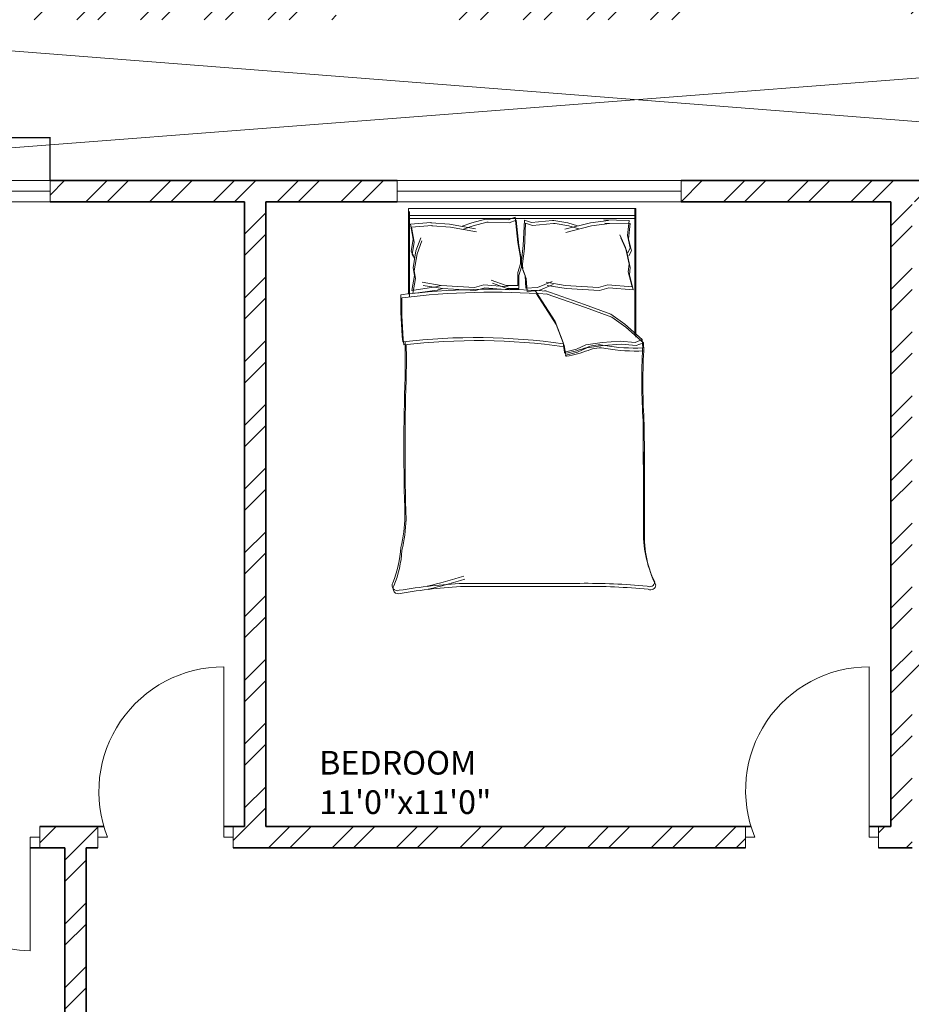
# Model space of a CAD drawing. Units: inches. Extents: x 1885 to 2748, y 783 to 2421.
# Tile 41 of 117: x 2098 to 2287, y 1350 to 1558. Entities that reach past the tile are written whole.
import ezdxf

# ---------------------------------------------------------------- set-up
doc = ezdxf.new("R2010")
doc.units = ezdxf.units.IN
for name, color, linetype, lineweight in [('A-ANNO-DIMS', 2, 'Continuous', 18), ('A-AREA-IDEN', 7, 'Continuous', 18), ('A-DOOR', 31, 'Continuous', 18), ('A-FLOR-OPEN', 8, 'Continuous', 13), ('A-FURN', 8, 'Continuous', 13), ('A-GLAZ', 181, 'Continuous', 18), ('A-WALL', 7, 'Continuous', 35)]:
    doc.layers.add(name, color=color, linetype=linetype, lineweight=lineweight)
doc.layers.add('A-WALL-PATT', color=85, linetype='Continuous', lineweight=13, true_color=0x58ba48)
doc.styles.get("Standard").update_dxf_attribs({"font": 'arial.ttf'})
doc.dimstyles.get("Standard").update_dxf_attribs({"dimtxt": 0.18, "dimasz": 0.18, "dimexe": 0.18, "dimexo": 0.0625, "dimgap": 0.09, "dimtad": 0, "dimtih": 1, "dimtoh": 1, "dimdec": 4, "dimzin": 0, "dimdsep": 46, "dimtxsty": 'Standard', "dimcen": 0.09, "dimadec": 0, "dimazin": 0, "dimtfac": 1, "dimtdec": 4, "dimtofl": 0, "dimtmove": 0, "dimatfit": 3, "dimfxl": 1, "dimtolj": 1, "dimtzin": 0, "dimarcsym": 0})

# ---------------------------------------------------------------- blocks, each defined once
blk = doc.blocks.new('BED-DOUBLE')
for p, q in [((27.75, 52.87), (24.5, 49.16)), ((27.75, 52.87), (24.5, 49.16)), ((28.39, 53.09), (25.14, 49.39)), ((28.39, 53.09), (25.14, 49.39)), ((29.49, 52.95), (27.75, 52.87, 3.87)), ((29.49, 52.95), (27.75, 52.87, 3.87)), ((28.37, 51.33), (27.75, 52.87)), ((28.37, 51.33), (27.75, 52.87)), ((30.13, 53.17), (28.39, 53.09, 3.87)), ((30.13, 53.17), (28.39, 53.09, 3.87)), ((29.01, 51.56), (28.39, 53.09)), ((29.01, 51.56), (28.39, 53.09)), ((0, 51.49), (0.64, 51.49)), ((0, 3.47), (0, 51.49)), ((0, 51.26), (26.61, 51.26)), ((0, 51.26), (26.61, 51.26)), ((0.64, 51.49), (27.25, 51.49)), ((0.64, 51.49), (27.25, 51.49)), ((1.54, 3.47), (1.54, 51.26)), ((1.54, 3.47), (1.54, 51.26)), ((2.18, 3.7), (2.18, 51.49)), ((2.18, 3.7), (2.18, 51.49)), ((2.56, 50.11), (2.46, 44.71)), ((2.56, 50.11), (2.46, 44.71)), ((2.56, 50.11), (5.77, 49.73)), ((2.56, 50.11), (5.77, 49.73)), ((3.2, 50.34), (3.1, 44.94)), ((3.2, 50.34), (3.1, 44.94)), ((3.2, 50.34), (6.41, 49.96)), ((3.2, 50.34), (6.41, 49.96)), ((5.77, 49.73), (8.34, 50.33)), ((5.77, 49.73), (8.34, 50.33)), ((6.41, 49.96), (8.98, 50.56)), ((6.41, 49.96), (8.98, 50.56)), ((11.83, 50.11), (8.26, 49.31)), ((11.83, 50.11), (8.26, 49.31)), ((8.34, 50.33), (9.39, 49.81)), ((8.34, 50.33), (9.39, 49.81)), ((12.47, 50.34), (8.9, 49.54)), ((12.47, 50.34), (8.9, 49.54)), ((8.98, 50.56), (10.03, 50.04)), ((8.98, 50.56), (10.03, 50.04)), ((13.44, 49.92), (11.83, 50.11)), ((13.44, 49.92), (11.83, 50.11)), ((14.08, 50.15), (12.47, 50.34)), ((14.08, 50.15), (12.47, 50.34)), ((16.58, 50.7), (13.44, 49.92)), ((16.58, 50.7), (13.44, 49.92)), ((17.22, 50.93), (14.08, 50.15)), ((17.22, 50.93), (14.08, 50.15)), ((16.17, 45.57), (16.58, 50.7)), ((16.17, 45.56), (16.58, 50.7)), ((16.81, 45.79), (17.22, 50.93)), ((16.81, 45.79), (17.22, 50.93)), ((28.06, 48.23), (28.37, 51.33)), ((28.06, 48.23), (28.37, 51.33)), ((28.7, 48.46), (29.01, 51.56)), ((28.7, 48.46), (29.01, 51.56)), ((8.26, 49.31), (5.58, 48.13)), ((8.26, 49.31), (5.58, 48.13)), ((8.9, 49.54), (6.22, 48.36)), ((8.9, 49.54), (6.22, 48.36)), ((24.5, 49.16), (22.33, 46.22)), ((24.5, 49.16), (22.33, 46.22)), ((25.14, 49.39), (22.97, 46.45)), ((25.14, 49.39), (22.97, 46.45)), ((28.37, 44.36), (28.06, 48.23)), ((28.37, 44.36), (28.06, 48.23)), ((29.01, 44.59), (28.7, 48.46)), ((29.01, 44.59), (28.7, 48.46)), ((3.1, 44.94), (3.19, 45.94)), ((3.1, 44.94), (3.19, 45.94)), ((3.19, 45.94), (3.71, 42.14)), ((3.19, 45.94), (3.71, 42.14)), ((17.37, 43.83), (16.81, 45.79)), ((17.37, 43.83), (16.81, 45.79)), ((22.33, 46.22), (20.32, 40.64)), ((22.33, 46.22), (20.32, 40.64)), ((22.97, 46.45), (20.96, 40.87)), ((22.97, 46.45), (20.96, 40.87)), ((2.46, 44.71), (2.55, 45.71)), ((2.46, 44.71), (2.55, 45.71)), ((2.55, 45.71), (3.07, 41.91)), ((2.55, 45.71), (3.07, 41.91)), ((16.73, 43.6), (16.17, 45.57)), ((16.73, 43.6), (16.17, 45.56)), ((16.94, 36.82), (17.37, 43.83)), ((16.94, 36.82), (17.37, 43.83)), ((28.83, 40.95), (28.37, 44.36)), ((28.83, 40.95), (28.37, 44.36)), ((29.47, 41.18), (29.01, 44.59)), ((29.47, 41.18), (29.01, 44.59)), ((3.07, 41.91), (4.43, 36.49)), ((3.07, 41.91), (4.43, 36.49)), ((3.71, 42.14), (5.07, 36.72)), ((3.71, 42.14), (5.07, 36.72)), ((16.3, 36.59), (16.73, 43.6)), ((16.3, 36.59), (16.73, 43.6)), ((20.32, 40.64), (17.39, 32.3)), ((20.32, 40.64), (17.39, 32.3)), ((20.96, 40.87), (18.03, 32.53)), ((20.96, 40.87), (18.03, 32.53)), ((29.76, 38.94), (28.83, 40.95)), ((29.76, 38.94), (28.83, 40.95)), ((30.4, 39.17), (29.47, 41.18)), ((30.4, 39.17), (29.47, 41.18)), ((79.25, 15.06), (79.25, 39.68)), ((79.25, 15.06), (79.25, 39.68)), ((79.89, 15.29), (79.89, 39.9)), ((79.89, 15.29), (79.89, 39.9)), ((3.68, 39.2), (3.08, 37.13)), ((3.68, 39.2), (3.08, 37.13)), ((4.32, 39.43), (3.72, 37.36)), ((4.32, 39.43), (3.72, 37.36)), ((30.38, 36.46), (29.76, 38.94)), ((30.38, 36.46), (29.76, 38.94)), ((31.02, 36.69), (30.4, 39.17)), ((31.02, 36.69), (30.4, 39.17)), ((3.08, 37.13), (2.54, 34.2)), ((3.08, 37.13), (2.54, 34.2)), ((3.72, 37.36), (3.18, 34.43)), ((3.72, 37.36), (3.18, 34.43)), ((15.63, 32.56), (16.3, 36.59)), ((15.63, 32.56), (16.3, 36.59)), ((16.27, 32.79), (16.94, 36.82)), ((16.27, 32.79), (16.94, 36.82)), ((23.88, 34.45), (28.37, 36.15)), ((23.88, 34.45), (28.37, 36.15)), ((24.52, 34.68), (29.01, 36.38)), ((24.52, 34.68), (29.01, 36.38)), ((28.37, 36.15), (30.38, 36.46)), ((28.37, 36.15), (30.38, 36.46)), ((29.01, 36.38), (31.02, 36.69)), ((29.01, 36.38), (31.02, 36.69)), ((2.54, 34.2), (2.56, 33.88)), ((2.54, 34.2), (2.56, 33.88)), ((2.56, 33.88), (2.98, 29.45)), ((2.56, 33.88), (2.98, 29.45)), ((3.18, 34.43), (3.2, 34.11)), ((3.18, 34.43), (3.2, 34.11)), ((3.2, 34.11), (3.62, 29.68)), ((3.2, 34.11), (3.62, 29.68)), ((16.74, 30.75), (15.46, 33.82)), ((16.74, 30.75), (15.46, 33.82)), ((17.38, 30.98), (16.1, 34.05)), ((17.38, 30.98), (16.1, 34.05)), ((17.39, 30.26), (23.88, 34.45)), ((17.39, 30.26), (23.88, 34.45)), ((18.03, 30.49), (24.52, 34.68)), ((18.03, 30.49), (24.52, 34.68)), ((2.98, 29.45), (2.5, 27.98)), ((2.98, 29.45), (2.5, 27.98)), ((3.62, 29.68), (3.13, 28.2)), ((3.62, 29.68), (3.13, 28.2)), ((16.9, 28.3), (16.74, 30.75)), ((16.9, 28.3), (16.74, 30.75)), ((17.54, 28.52), (17.38, 30.98)), ((17.54, 28.52), (17.38, 30.98)), ((2.5, 27.98), (7.87, 27.73)), ((2.5, 27.98), (7.87, 27.73)), ((3.13, 28.2), (8.51, 27.96)), ((3.13, 28.2), (8.51, 27.96)), ((7.22, 26.56), (10.4, 27.14)), ((7.22, 26.56), (10.4, 27.14)), ((7.86, 26.79), (11.04, 27.37)), ((7.86, 26.79), (11.04, 27.37)), ((7.87, 27.73), (11.08, 27.35)), ((7.87, 27.73), (11.08, 27.35)), ((8.51, 27.96), (11.72, 27.58)), ((8.51, 27.96), (11.72, 27.58)), ((10.4, 27.14), (11.71, 27.14)), ((10.4, 27.14), (11.71, 27.14)), ((11.04, 27.37), (12.35, 27.37)), ((11.04, 27.37), (12.35, 27.37)), ((11.08, 27.35), (12.38, 27.43)), ((11.08, 27.35), (12.38, 27.43)), ((11.71, 27.14), (13.59, 26.56)), ((11.71, 27.14), (13.59, 26.56)), ((11.72, 27.58), (13.02, 27.66)), ((11.72, 27.58), (13.02, 27.66)), ((12.35, 27.37), (14.22, 26.79)), ((12.35, 27.37), (14.22, 26.79)), ((12.38, 27.43), (14.22, 28.13)), ((12.38, 27.43), (14.22, 28.13)), ((13.02, 27.66), (14.86, 28.36)), ((13.02, 27.66), (14.86, 28.36)), ((14.22, 28.13), (16.9, 28.3)), ((14.22, 28.13), (16.9, 28.3)), ((14.86, 28.36), (17.54, 28.52)), ((14.86, 28.36), (17.54, 28.52)), ((1.87, 25.98), (7.22, 26.56)), ((1.87, 25.98), (7.22, 26.56)), ((2.45, 24.54), (1.87, 25.98)), ((2.45, 24.54), (1.87, 25.98)), ((2.51, 26.21), (7.86, 26.79)), ((2.51, 26.21), (7.86, 26.79)), ((3.09, 24.76), (2.51, 26.21)), ((3.09, 24.76), (2.51, 26.21)), ((13.59, 26.56), (16.27, 26.56)), ((13.59, 26.56), (16.27, 26.56)), ((14.22, 26.79), (16.91, 26.79)), ((14.22, 26.79), (16.91, 26.79)), ((16.27, 26.56), (16.27, 24.1)), ((16.27, 26.56), (16.27, 24.1)), ((16.91, 26.79), (16.91, 24.33)), ((16.91, 26.79), (16.91, 24.33)), ((2.31, 20.09), (2.45, 24.54)), ((2.31, 20.09), (2.45, 24.54)), ((2.95, 20.32), (3.09, 24.76)), ((2.95, 20.32), (3.09, 24.76)), ((16.27, 24.1), (15.18, 20.96)), ((16.27, 24.1), (15.18, 20.96)), ((16.91, 24.33), (15.82, 21.19)), ((16.91, 24.33), (15.82, 21.19)), ((16.17, 19.38), (16.58, 24.51)), ((16.17, 19.38), (16.58, 24.51)), ((16.81, 19.61), (17.22, 24.74)), ((16.81, 19.61), (17.22, 24.74)), ((2.31, 19.77), (2.31, 20.09)), ((2.31, 19.77), (2.31, 20.09)), ((3.03, 16.88), (2.31, 19.77)), ((3.03, 16.88), (2.31, 19.77)), ((2.95, 20), (2.95, 20.32)), ((2.95, 20), (2.95, 20.32)), ((3.67, 17.11), (2.95, 20)), ((3.67, 17.11), (2.95, 20)), ((16.73, 17.42), (16.17, 19.38)), ((16.73, 17.42), (16.17, 19.38)), ((17.37, 17.65), (16.81, 19.61)), ((17.37, 17.65), (16.81, 19.61)), ((3.75, 14.85), (3.03, 16.88)), ((3.75, 14.85), (3.03, 16.88)), ((3.32, 12.11), (4.33, 17.6)), ((3.32, 12.11), (4.33, 17.6)), ((4.39, 15.08), (3.67, 17.11)), ((4.39, 15.08), (3.67, 17.11)), ((3.96, 12.34), (4.97, 17.83)), ((3.96, 12.34), (4.97, 17.83)), ((16.3, 10.41), (16.73, 17.42)), ((16.3, 10.41), (16.73, 17.42)), ((16.94, 10.64), (17.37, 17.65)), ((16.94, 10.64), (17.37, 17.65)), ((3.03, 8.28), (3.32, 12.11)), ((3.03, 8.28), (3.32, 12.11)), ((3.67, 8.51), (3.96, 12.34)), ((3.67, 8.51), (3.96, 12.34)), ((15.63, 6.38), (16.3, 10.41)), ((15.63, 6.38), (16.3, 10.41)), ((16.27, 6.61), (16.94, 10.64)), ((16.27, 6.61), (16.94, 10.64)), ((16.3, 10.41), (16.62, 9.28)), ((16.3, 10.41), (16.62, 9.28)), ((16.94, 10.64), (17.26, 9.51)), ((16.94, 10.64), (17.26, 9.51)), ((3.65, 8.41), (3.67, 8.51)), ((3.65, 8.41), (3.67, 8.51)), ((3.98, 4.13), (3.65, 8.41)), ((3.98, 4.13), (3.65, 8.41)), ((16.62, 9.28), (17.34, 4.18)), ((16.62, 9.28), (17.34, 4.18)), ((17.26, 9.51), (17.98, 4.41)), ((17.26, 9.51), (17.98, 4.41)), ((3.01, 8.18), (3.03, 8.28)), ((3.01, 8.18), (3.03, 8.28)), ((3.34, 3.9), (3.01, 8.18)), ((3.34, 3.9), (3.01, 8.18)), ((9.6, 5.28), (6.85, 6.29)), ((9.6, 5.28), (6.85, 6.29)), ((3.32, 3.89), (6.5, 4.47)), ((3.32, 3.89), (6.5, 4.47)), ((3.96, 4.12), (7.14, 4.7)), ((3.96, 4.12), (7.14, 4.7)), ((8.96, 5.05), (6.21, 6.06)), ((8.96, 5.05), (6.21, 6.06)), ((6.5, 4.47), (9.1, 4.04)), ((6.5, 4.47), (9.1, 4.04)), ((7.14, 4.7), (9.74, 4.27)), ((7.14, 4.7), (9.74, 4.27)), ((12.57, 4.47), (8.96, 5.05)), ((12.57, 4.47), (8.96, 5.05)), ((9.1, 4.04), (10.12, 4.62)), ((9.1, 4.04), (10.12, 4.62)), ((13.21, 4.7), (9.6, 5.28)), ((13.21, 4.7), (9.6, 5.28)), ((9.74, 4.27), (10.75, 4.84)), ((9.74, 4.27), (10.75, 4.84)), ((14.16, 4.76), (12.57, 4.47)), ((14.16, 4.76), (12.57, 4.47)), ((14.8, 4.99), (13.21, 4.7)), ((14.8, 4.99), (13.21, 4.7)), ((17.34, 4.18), (14.16, 4.76)), ((17.34, 4.18), (14.16, 4.76)), ((17.98, 4.41), (14.8, 4.99)), ((17.98, 4.41), (14.8, 4.99)), ((18.11, 3.47), (0, 3.47)), ((18.11, 3.47), (0, 3.47)), ((18.75, 3.7), (0.64, 3.7)), ((18.75, 3.7), (0.64, 3.7))]:
    blk.add_line(p, q)
for centre, radius, start, end in [((68.67, 76.16), 23.07, 267.4714, 296.4681), ((68.67, 76.16), 23.07, 267.4714, 296.4681), ((69.31, 76.38), 23.07, 267.4714, 296.4681), ((69.31, 76.38), 23.07, 267.4714, 296.4681), ((78.87, 54.41), 1.1, 332.6588, 86.02), ((78.87, 54.41), 1.1, 332.6588, 86.02), ((79.51, 54.64), 1.1, 332.6588, 86.02), ((79.51, 54.64), 1.1, 332.6588, 86.02), ((212.92, 41.38), 133.04, 174.4998, 180.6351), ((212.92, 41.38), 133.04, 174.4998, 180.6351), ((-6.65, 51.33), 36.18, 349.8763, 2.5657), ((-6.65, 51.33), 36.18, 349.8763, 2.5657), ((36.32, 182.26), 129.5, 266.9791, 273.8365), ((36.32, 182.26), 129.5, 266.9791, 273.8365), ((-6.01, 51.55), 36.18, 349.8763, 2.5657), ((-6.01, 51.55), 36.18, 349.8763, 2.5657), ((36.96, 182.49), 129.5, 266.9791, 273.8365), ((36.96, 182.49), 129.5, 266.9791, 273.8365), ((67.83, -4508.74), 4561.86, 90.00217, 90.28689), ((67.83, -4508.75), 4561.86, 90.00217, 90.28689), ((68.46, -4508.52), 4561.86, 90.00217, 90.28689), ((68.46, -4508.52), 4561.86, 90.00217, 90.28689), ((212.28, 41.15), 133.04, 174.4998, 180.6351), ((212.28, 41.15), 133.04, 174.4998, 180.6351), ((35.07, 43.74), 6.22, 168.6608, 203.7384), ((35.07, 43.74), 6.22, 168.6608, 203.7384), ((35.71, 43.97), 6.22, 168.6608, 203.7384), ((35.71, 43.97), 6.22, 168.6608, 203.7384), ((1.49, 31.15), 29.65, 10.6617, 19.8806), ((1.49, 31.15), 29.65, 10.6617, 19.8806), ((2.13, 31.38), 29.65, 10.6617, 19.8806), ((2.13, 31.38), 29.65, 10.6617, 19.8806), ((156.32, 17.75), 129.02, 171.7845, 186.9006), ((156.32, 17.75), 129.02, 171.7845, 186.9006), ((156.96, 17.98), 129.02, 171.7845, 186.9006), ((156.96, 17.98), 129.02, 171.7845, 186.9006), ((30.44, 36.64), 0.185, 250.2464, 1.1377), ((30.44, 36.63), 0.185, 250.2464, 1.1377), ((31.08, 36.86), 0.185, 250.2464, 1.1377), ((31.08, 36.86), 0.185, 250.2464, 1.1377), ((182.06, 21.36), 164.97, 176.0865, 186.7821), ((182.06, 21.36), 164.97, 176.0865, 186.7821), ((182.7, 21.59), 164.97, 176.0865, 186.7821), ((182.7, 21.59), 164.97, 176.0865, 186.7821), ((-23.71, -17.22), 106.46, 13.3832, 17.7053), ((-23.71, -17.22), 106.46, 13.3832, 17.7053), ((-23.07, -16.99), 106.46, 13.3832, 17.7053), ((-23.07, -16.99), 106.46, 13.3832, 17.7053), ((200.84, 21.43), 121.76, 182.9958, 189.4091), ((200.84, 21.43), 121.76, 182.9958, 189.4091), ((201.48, 21.65), 121.76, 182.9958, 189.4091), ((201.48, 21.65), 121.76, 182.9958, 189.4091), ((20.1, 85.16), 83.31, 268.7218, 275.604), ((20.1, 85.16), 83.31, 268.7218, 275.604), ((20.74, 85.39), 83.31, 268.7218, 275.604), ((20.74, 85.39), 83.31, 268.7218, 275.604), ((31.18, -167.31), 170.11, 88.4762, 91.0082), ((31.18, -167.31), 170.11, 88.4762, 91.0082), ((31.82, -167.08), 170.11, 88.4762, 91.0082), ((31.82, -167.08), 170.11, 88.4762, 91.0082), ((50.62, 484.82), 482.31, 268.2277, 271.7185), ((50.62, 484.82), 482.31, 268.2277, 271.7185), ((51.26, 485.05), 482.31, 268.2277, 271.7185), ((51.26, 485.05), 482.31, 268.2277, 271.7185), ((64.52, -26.9), 29.63, 76.0648, 88.9113), ((64.52, -26.9), 29.63, 76.0648, 88.9113), ((65.16, -26.67), 29.63, 76.0648, 88.9113), ((65.16, -26.67), 29.63, 76.0648, 88.9113), ((70.92, -21.43), 23.56, 67.9751, 86.652), ((70.92, -21.43), 23.56, 67.9751, 86.652), ((70.28, -21.66), 23.56, 67.9751, 86.652), ((70.28, -21.66), 23.56, 67.9751, 86.652), ((79.72, 1.09), 1.09, 236.1736, 23.4781), ((79.72, 1.09), 1.09, 236.1736, 23.4781), ((80.36, 1.31), 1.09, 236.1736, 23.4781), ((80.36, 1.31), 1.09, 236.1736, 23.4781)]:
    blk.add_arc(centre, radius, start, end)
blk = doc.blocks.new('WIN-60')
for p, q in [((0, 60), (4.5, 60)), ((0, 60), (0, 0)), ((4.5, 60), (2.25, 60)), ((2.25, 60), (2.25, 0)), ((4.5, 0), (4.5, 60)), ((2.25, 0), (0, 0)), ((0, 0), (4.5, 0))]:
    blk.add_line(p, q)
blk = doc.blocks.new('*D15')
at = {"layer": 'A-ANNO-DIMS', "color": 0, "lineweight": -2, "transparency": 16777216}
for p, q in [((2044.67, 1524.07), (2044.67, 1533.19)), ((2044.85, 1533.01), (2073.56, 1533.01)), ((2104.49, 1533.01), (2075.79, 1533.01)), ((2104.67, 1524.07), (2104.67, 1533.19))]:
    blk.add_line(p, q, dxfattribs=at)
at = {"layer": 'A-ANNO-DIMS', "color": 0, "transparency": 16777216}
for points in [[(2044.85, 1533.04), (2044.85, 1532.98), (2044.67, 1533.01)], [(2104.49, 1533.04), (2104.49, 1532.98), (2104.67, 1533.01)]]:
    blk.add_solid(points, dxfattribs=at)
at = {"layer": 'Defpoints', "color": 0, "transparency": 16777216}
for p in [(2104.67, 1533.01), (2044.67, 1524.01), (2104.67, 1524.01)]:
    blk.add_point(p, dxfattribs=at)
at = {"layer": 'A-ANNO-DIMS', "color": 0, "transparency": 16777216, "insert": (2074.67, 1533.01), "char_height": 0.18, "attachment_point": 5}
blk.add_mtext('\\A1;WINDOW 60 TYP.', dxfattribs=at)

msp = doc.modelspace()

# ---------------------------------------------------------------- hatches: boundary and pattern name
at = {"layer": 'A-WALL-PATT'}
h = msp.add_hatch(dxfattribs=at)
h.set_pattern_fill('ANSI32', color=256)
h.paths.add_polyline_path([(2007.77, 2318.01), (1980.77, 2318.01), (1980.77, 2281.22), (1985.27, 2281.22), (1985.27, 2313.51), (2007.77, 2313.51), (2007.77, 2315.76)])
h.paths.add_polyline_path([(2094.32, 2318.01), (2067.77, 2318.01), (2067.77, 2313.51), (2094.32, 2313.51), (2094.32, 2315.76)])
h.paths.add_polyline_path([(2131.37, 2315.76), (2131.37, 2318.01), (2131.19, 2318.01), (2112.61, 2318.01), (2112.61, 2313.51), (2117.27, 2313.51), (2117.27, 2255.2), (2121.77, 2255.2), (2121.77, 2313.51), (2131.37, 2313.51)])
h.paths.add_polyline_path([(2190.51, 2318.01), (2155.37, 2318.01), (2155.37, 2313.51), (2169.77, 2313.51), (2169.77, 2229.51), (2121.77, 2229.51), (2121.77, 2233.45), (2119.52, 2233.45), (2117.27, 2233.45), (2117.27, 2201.1), (2121.77, 2201.1), (2121.77, 2225.01), (2169.77, 2225.01), (2169.77, 2165.01), (2306.27, 2165.01), (2306.27, 2066.01), (2310.77, 2066.01), (2344.27, 2066.01), (2486.27, 2066.01), (2486.27, 1886.01), (2483.02, 1886.01), (2483.02, 1881.51), (2486.27, 1881.51), (2486.27, 1880.68), (2490.77, 1880.68), (2490.77, 2070.51), (2344.27, 2070.51), (2310.77, 2070.51), (2310.77, 2165.01), (2310.77, 2173.64), (2308.52, 2173.64), (2306.27, 2173.64), (2306.27, 2169.51), (2174.27, 2169.51), (2174.27, 2313.51), (2190.51, 2313.51), (2190.51, 2315.76)])
h.paths.add_polyline_path([(1985.27, 2221.22), (1980.77, 2221.22), (1980.77, 2165.01), (1992.77, 2165.01), (1992.77, 2141.93), (1997.27, 2141.93), (1997.27, 2165.01), (2117.27, 2165.01), (2117.27, 2163.13), (2121.77, 2163.13), (2121.77, 2172.73), (2119.52, 2172.73), (2117.27, 2172.73), (2117.27, 2169.51), (1985.27, 2169.51)])
h.paths.add_polyline_path([(1997.27, 2105.93), (1992.77, 2105.93), (1992.77, 2070.51), (2016.77, 2070.51), (2016.77, 2059.12), (2019.02, 2059.12), (2021.27, 2059.12), (2021.27, 2070.51), (2117.27, 2070.51), (2117.27, 2022.51), (2114.42, 2022.51), (2114.42, 2018.01), (2123.63, 2018.01), (2123.63, 2020.26), (2123.63, 2022.51), (2121.77, 2022.51), (2121.77, 2142.59), (2119.52, 2142.59), (2117.27, 2142.59), (2117.27, 2075.01), (1997.27, 2075.01)])
h.paths.add_polyline_path([(2092.03, 2020.26), (2092.03, 2022.51), (2021.27, 2022.51), (2021.27, 2035.12), (2016.77, 2035.12), (2016.77, 2018.01), (2016.77, 1978.78), (2021.27, 1978.78), (2021.27, 2018.01), (2092.03, 2018.01)])
h.paths.add_polyline_path([(2260.94, 2022.51), (2153.1, 2022.51), (2153.1, 2020.26), (2153.1, 2018.01), (2155.27, 2018.01), (2155.27, 1886.01), (2107.63, 1886.01), (2107.63, 1881.51), (2182.91, 1881.51), (2182.91, 1883.76), (2182.91, 1886.01), (2159.77, 1886.01), (2159.77, 2018.01), (2260.94, 2018.01), (2260.94, 2020.26)])
h.paths.add_polyline_path([(2047.63, 1883.76), (2047.63, 1886.01), (2021.27, 1886.01), (2021.27, 1918.78), (2019.02, 1918.78), (2016.77, 1918.78), (2016.77, 1881.51), (2047.63, 1881.51)])
h.paths.add_polyline_path([(2306.36, 1883.76), (2306.36, 1886.01), (2296.27, 1886.01), (2296.27, 1982.01), (2316.54, 1982.01), (2316.54, 1984.26), (2316.54, 1986.51), (2296.27, 1986.51), (2296.27, 2022.51), (2289.28, 2022.51), (2289.28, 2018.01), (2291.77, 2018.01), (2291.77, 1886.01), (2242.91, 1886.01), (2242.91, 1881.51), (2306.36, 1881.51)], flags=17)
h.paths.add_polyline_path([(1985.27, 1843.01), (2021.6, 1843.01), (2021.53, 1845.44), (2021.48, 1847.51), (1980.77, 1847.51), (1980.77, 1809.45), (1985.27, 1809.45)])
h.paths.add_polyline_path([(2131.48, 1845.26), (2131.48, 1847.51), (2081.53, 1847.51), (2081.53, 1843.01), (2117.27, 1843.01), (2117.27, 1784.15), (2119.52, 1784.15), (2121.77, 1784.15), (2121.77, 1843.01), (2131.48, 1843.01)])
h.paths.add_polyline_path([(2203.89, 1847.51), (2155.48, 1847.51), (2155.48, 1843.01), (2169.77, 1843.01), (2169.77, 1759.01), (2121.77, 1759.01), (2121.77, 1761.46), (2117.27, 1761.46), (2117.27, 1730.43), (2121.77, 1730.43), (2121.77, 1754.51), (2177.42, 1754.51), (2177.42, 1756.76), (2177.42, 1759.01), (2174.27, 1759.01), (2174.27, 1843.01), (2203.89, 1843.01)])
h.paths.add_polyline_path([(2335.55, 1845.26), (2335.55, 1847.51), (2239.89, 1847.51), (2239.89, 1843.01), (2306.27, 1843.01), (2306.27, 1759.01), (2199.49, 1759.01), (2199.49, 1754.51), (2310.77, 1754.51), (2310.77, 1843.01), (2335.55, 1843.01)])
h.paths.add_polyline_path([(2348.77, 2022.51), (2344.27, 2022.51), (2344.27, 1986.51), (2341.68, 1986.51), (2341.68, 1982.01), (2344.27, 1982.01), (2344.27, 1886.01), (2330.36, 1886.01), (2330.36, 1881.51), (2361.63, 1881.51), (2361.63, 1883.76), (2361.63, 1886.01), (2348.77, 1886.01)], flags=17)
h.paths.add_polyline_path([(2283.25, 2315.76), (2283.25, 2318.01), (2238.51, 2318.01), (2238.51, 2313.51), (2283.25, 2313.51)], flags=17)
h.paths.add_polyline_path([(2363.27, 2348.01), (2388.68, 2348.01), (2388.68, 2350.26), (2388.68, 2352.51), (2358.77, 2352.51), (2358.77, 2348.01), (2358.77, 2318.01), (2344.48, 2318.01), (2344.48, 2313.51), (2358.77, 2313.51), (2358.77, 2229.51), (2310.77, 2229.51), (2310.77, 2231.95), (2306.27, 2231.95), (2306.27, 2205.61), (2310.77, 2205.61), (2310.77, 2225.01), (2358.77, 2225.01), (2358.77, 2211.51), (2452.33, 2211.51), (2452.33, 2213.76), (2452.33, 2216.01), (2363.27, 2216.01), (2363.27, 2318.01)])
h.paths.add_polyline_path([(2310.77, 2313.51), (2320.48, 2313.51), (2320.48, 2315.76), (2320.48, 2318.01), (2302.73, 2318.01), (2302.73, 2313.51), (2306.27, 2313.51), (2306.27, 2251.08), (2310.77, 2251.08)], flags=17)
h.paths.add_polyline_path([(2490.77, 2352.51), (2486.27, 2352.51), (2448.68, 2352.51), (2448.68, 2348.01), (2486.27, 2348.01), (2486.27, 2318.01), (2486.27, 2216.01), (2481.78, 2216.01), (2481.78, 2211.51), (2486.27, 2211.51), (2486.27, 2165.01), (2493.29, 2165.01), (2493.29, 2167.26), (2493.29, 2169.51), (2490.77, 2169.51), (2490.77, 2313.51), (2494.43, 2313.51), (2494.43, 2318.01), (2490.77, 2318.01)])
h.paths.add_polyline_path([(2534.65, 2318.01), (2515.69, 2318.01), (2515.69, 2313.51), (2534.65, 2313.51), (2534.65, 2315.76)])
h.paths.add_polyline_path([(2618.27, 2318.01), (2594.65, 2318.01), (2594.65, 2313.51), (2613.77, 2313.51), (2613.77, 2281.71), (2618.27, 2281.71)])
h.paths.add_polyline_path([(2618.27, 2221.71), (2613.77, 2221.71), (2613.77, 2169.51), (2554.02, 2169.51), (2554.02, 2165.01), (2613.77, 2165.01), (2613.77, 2152.88), (2618.27, 2152.88)])
h.paths.add_polyline_path([(2618.27, 2128.88), (2616.02, 2128.88), (2613.77, 2128.88), (2613.77, 2117.01), (2529.77, 2117.01), (2529.77, 2165.01), (2532.85, 2165.01), (2532.85, 2169.51), (2522.87, 2169.51), (2522.87, 2165.01), (2525.27, 2165.01), (2525.27, 2117.01), (2525.27, 2112.51), (2525.27, 2108.58), (2529.77, 2108.58), (2529.77, 2112.51), (2613.77, 2112.51), (2613.77, 2080.19), (2618.27, 2080.19)])
h.paths.add_polyline_path([(2618.27, 2044.19), (2616.02, 2044.19), (2613.77, 2044.19), (2613.77, 2015.51), (2529.77, 2015.51), (2529.77, 2088.58), (2527.52, 2088.58), (2525.27, 2088.58), (2525.27, 2011.01), (2613.77, 2011.01), (2613.77, 1956.75), (2618.27, 1956.75)])
h.paths.add_polyline_path([(2618.27, 1881.51), (2618.27, 1896.75), (2613.77, 1896.75), (2613.77, 1881.51), (2613.77, 1847.51), (2592.71, 1847.51), (2592.71, 1843.01), (2613.77, 1843.01), (2613.77, 1765.01), (2613.77, 1760.51), (2609.62, 1760.51), (2609.62, 1756.01), (2613.77, 1756.01), (2613.77, 1660.01), (2608.54, 1660.01), (2608.54, 1655.51), (2613.77, 1655.51), (2613.77, 1508.16), (2618.27, 1508.16)])
h.paths.add_polyline_path([(2565.77, 1843.01), (2569, 1843.01), (2569, 1847.51), (2490.77, 1847.51), (2490.77, 1849.7), (2488.52, 1849.7), (2486.27, 1849.7), (2486.27, 1847.51), (2477.27, 1847.51), (2477.27, 1838.51), (2477.27, 1821.49), (2486.27, 1821.49), (2486.27, 1838.51), (2561.27, 1838.51), (2561.27, 1765.01), (2486.27, 1765.01), (2486.27, 1786.16), (2477.27, 1786.16), (2477.27, 1765.01), (2477.27, 1756.01), (2486.27, 1756.01), (2565.77, 1756.01), (2585.62, 1756.01), (2585.62, 1758.26), (2585.62, 1760.51), (2565.77, 1760.51), (2565.77, 1765.01)])
h.paths.add_polyline_path([(2486.27, 1651.01), (2561.27, 1651.01), (2561.27, 1567.01), (2486.27, 1567.01), (2486.27, 1591.32), (2477.27, 1591.32), (2477.27, 1567.01), (2477.27, 1558.01), (2477.27, 1555.44), (2481.77, 1555.44), (2481.77, 1558.01), (2568.65, 1558.01), (2568.65, 1560.26), (2568.65, 1562.51), (2565.77, 1562.51), (2565.77, 1655.51), (2584.54, 1655.51), (2584.54, 1657.76), (2584.54, 1660.01), (2565.77, 1660.01), (2486.27, 1660.01), (2477.27, 1660.01), (2477.27, 1651.01), (2477.27, 1632.99), (2486.27, 1632.99)])
h.paths.add_polyline_path([(2449.97, 1883.76), (2449.97, 1886.01), (2421.63, 1886.01), (2421.63, 1881.51), (2449.97, 1881.51)], flags=17)
h.paths.add_polyline_path([(2447.27, 1847.51), (2395.55, 1847.51), (2395.55, 1843.01), (2442.77, 1843.01), (2442.77, 1809.27), (2447.27, 1809.27)])
h.paths.add_polyline_path([(1985.27, 1749.45), (1980.77, 1749.45), (1980.77, 1694.5), (1985.27, 1694.5), (1985.27, 1694.51), (1986.9, 1694.51), (1986.9, 1697.78), (1986.9, 1699.01), (1985.27, 1699.01)])
h.paths.add_polyline_path([(2152.77, 1699.01), (2121.77, 1699.01), (2121.77, 1703.67), (2119.52, 1703.67), (2117.27, 1703.67), (2117.27, 1699.01), (2009.22, 1699.01), (2009.22, 1694.51), (2148.27, 1694.51), (2148.27, 1692.63), (2152.77, 1692.63)])
h.paths.add_polyline_path([(2016.27, 1694.51), (2011.77, 1694.51), (2011.77, 1558.01), (2040.81, 1558.01), (2040.81, 1560.26), (2040.81, 1562.51), (2016.27, 1562.51)])
h.paths.add_polyline_path([(2152.77, 1663.02), (2150.52, 1663.02), (2148.27, 1663.02), (2148.27, 1562.51), (2100.81, 1562.51), (2100.81, 1558.01), (2165.12, 1558.01), (2165.12, 1560.26), (2165.12, 1562.51), (2152.77, 1562.51), (2152.77, 1610.51), (2224.77, 1610.51), (2224.77, 1607.99), (2229.27, 1607.99), (2229.27, 1615.01), (2152.77, 1615.01)])
h.paths.add_polyline_path([(2238.61, 1560.26), (2238.61, 1562.51), (2229.27, 1562.51), (2229.27, 1588.76), (2227.02, 1588.76), (2224.77, 1588.77), (2224.77, 1562.51), (2189.12, 1562.51), (2189.12, 1558.01), (2238.61, 1558.01)])
h.paths.add_polyline_path([(2336.02, 1560.26), (2336.02, 1562.51), (2310.77, 1562.51), (2310.77, 1656.35), (2308.52, 1656.35), (2306.27, 1656.35), (2306.27, 1562.51), (2286.61, 1562.51), (2286.61, 1558.01), (2336.02, 1558.01)])
h.paths.add_polyline_path([(2447.27, 1690.97), (2445.02, 1690.97), (2442.77, 1690.97), (2442.77, 1687.01), (2306.27, 1687.01), (2306.27, 1680.75), (2310.77, 1680.75), (2310.77, 1682.51), (2442.77, 1682.51), (2442.77, 1562.51), (2396.02, 1562.51), (2396.02, 1558.01), (2447.27, 1558.01)])
h.paths.add_polyline_path([(2447.27, 1749.27), (2445.02, 1749.27), (2442.77, 1749.27), (2442.77, 1717.23), (2447.27, 1717.23)])
h.paths.add_polyline_path([(2044.67, 1521.76), (2044.67, 1524.01), (2007.27, 1524.01), (2007.27, 1503.49), (2009.52, 1503.49), (2011.77, 1503.49), (2011.77, 1519.51), (2044.67, 1519.51)])
h.paths.add_polyline_path([(2177.97, 1521.76), (2177.97, 1524.01), (2104.67, 1524.01), (2104.67, 1519.51), (2145.77, 1519.51), (2145.77, 1387.51), (2143.37, 1387.51), (2143.37, 1383.01), (2251.59, 1383.01), (2251.59, 1385.26), (2251.59, 1387.51), (2150.27, 1387.51), (2150.27, 1519.51), (2177.97, 1519.51)])
h.paths.add_polyline_path([(2298.7, 1524.01), (2237.97, 1524.01), (2237.97, 1519.51), (2282.27, 1519.51), (2282.27, 1387.51), (2279.68, 1387.51), (2279.68, 1383.01), (2286.77, 1383.01), (2286.77, 1419.01), (2312.45, 1419.01), (2312.45, 1421.26), (2312.45, 1423.51), (2286.77, 1423.51), (2286.77, 1519.51), (2298.7, 1519.51), (2298.7, 1521.72)], flags=17)
h.paths.add_polyline_path([(2361.9, 1521.76), (2361.9, 1524.01), (2322.7, 1524.01), (2322.7, 1519.51), (2334.77, 1519.51), (2334.77, 1423.51), (2331.93, 1423.51), (2331.93, 1419.01), (2334.77, 1419.01), (2334.77, 1387.51), (2334.77, 1383.23), (2339.27, 1383.23), (2339.27, 1387.51), (2339.27, 1519.51), (2361.9, 1519.51)], flags=17)
h.paths.add_polyline_path([(2447.27, 1521.76), (2447.27, 1524.01), (2421.9, 1524.01), (2421.9, 1519.51), (2447.27, 1519.51)], flags=17)
h.paths.add_polyline_path([(2481.77, 1529.6), (2479.52, 1529.6), (2477.27, 1529.6), (2477.27, 1524.01), (2474.49, 1524.01), (2474.49, 1519.51), (2477.27, 1519.51), (2477.27, 1334.51), (2296.77, 1334.51), (2296.77, 1240.51), (2160.27, 1240.51), (2160.27, 1180.51), (2112.27, 1180.51), (2112.27, 1207.69), (2110.02, 1207.69), (2107.77, 1207.69), (2107.77, 1171.61), (2112.27, 1171.61), (2112.27, 1176.01), (2160.27, 1176.01), (2160.27, 1092.01), (2144.22, 1092.01), (2144.22, 1087.51), (2189.5, 1087.51), (2189.5, 1089.76), (2189.5, 1092.01), (2164.77, 1092.01), (2164.77, 1236.01), (2296.77, 1236.01), (2296.77, 1231.91), (2301.27, 1231.91), (2301.27, 1330.01), (2481.77, 1330.01), (2481.77, 1387.51)])
h.paths.add_polyline_path([(2618.27, 1448.16), (2613.77, 1448.16), (2613.77, 1382.51), (2529.77, 1382.51), (2525.27, 1382.51), (2525.27, 1307.06), (2529.77, 1307.06), (2529.77, 1378.01), (2613.77, 1378.01), (2613.77, 1354.99), (2618.27, 1354.99)])
h.paths.add_polyline_path([(2618.27, 1318.99), (2613.77, 1318.99), (2613.77, 1281.01), (2529.77, 1281.01), (2529.77, 1283.79), (2527.52, 1283.79), (2525.27, 1283.79), (2525.27, 1228.51), (2516.79, 1228.51), (2516.79, 1224.01), (2533.48, 1224.01), (2533.48, 1226.26), (2533.48, 1228.51), (2529.77, 1228.51), (2529.77, 1276.51), (2613.77, 1276.51), (2613.77, 1266.02), (2618.27, 1266.02)])
h.paths.add_polyline_path([(2618.27, 1134.96), (2613.77, 1134.96), (2613.77, 1092.01), (2594.54, 1092.01), (2594.54, 1087.51), (2618.27, 1087.51)])
h.paths.add_polyline_path([(2534.54, 1092.01), (2509.77, 1092.01), (2509.77, 1087.51), (2534.54, 1087.51), (2534.54, 1089.76)])
h.paths.add_polyline_path([(2481.27, 1224.01), (2484.12, 1224.01), (2484.12, 1226.26), (2484.12, 1228.51), (2476.77, 1228.51), (2476.77, 1198.51), (2471.61, 1198.51), (2471.61, 1194.01), (2476.77, 1194.01), (2476.77, 1062.01), (2436.89, 1062.01), (2436.89, 1057.51), (2476.77, 1057.51), (2481.27, 1057.51), (2481.27, 1062.01), (2481.27, 1087.51), (2485.35, 1087.51), (2485.35, 1089.76), (2485.35, 1092.01), (2481.27, 1092.01), (2481.27, 1117.51)])
h.paths.add_polyline_path([(2439.9, 1198.51), (2349.27, 1198.51), (2349.27, 1194.01), (2349.27, 1180.51), (2301.27, 1180.51), (2301.27, 1201.9), (2299.02, 1201.9), (2296.77, 1201.9), (2296.77, 1172.34), (2299.02, 1172.34), (2301.27, 1172.34), (2301.27, 1176.01), (2349.27, 1176.01), (2349.27, 1092.01), (2334.45, 1092.01), (2334.45, 1087.51), (2349.27, 1087.51), (2349.27, 1057.51), (2353.77, 1057.51), (2376.89, 1057.51), (2376.89, 1059.76), (2376.89, 1062.01), (2353.77, 1062.01), (2353.77, 1087.51), (2353.77, 1180.51), (2353.77, 1194.01), (2439.9, 1194.01), (2439.9, 1196.26)])
h.paths.add_polyline_path([(2270.6, 1089.76), (2270.6, 1092.01), (2249.5, 1092.01), (2249.5, 1087.51), (2270.6, 1087.51)], flags=17)
h.paths.add_polyline_path([(2310.45, 1092.01), (2301.27, 1092.01), (2301.27, 1153.29), (2296.77, 1153.29), (2296.77, 1092.01), (2293.79, 1092.01), (2293.79, 1087.51), (2310.45, 1087.51), (2310.45, 1089.76)], flags=17)
h.paths.add_polyline_path([(2112.27, 1150.33), (2110.02, 1150.33), (2107.77, 1150.33), (2107.77, 1092.01), (2104.47, 1092.01), (2104.47, 1087.51), (2120.22, 1087.51), (2120.22, 1089.76), (2120.22, 1092.01), (2112.27, 1092.01)])
h.paths.add_polyline_path([(2082.17, 1092.01), (2058.14, 1092.01), (2058.14, 1087.51), (2082.17, 1087.51), (2082.17, 1089.76)])
h.paths.add_polyline_path([(1975.77, 1145.64), (1971.27, 1145.64), (1971.27, 1087.51), (1980.77, 1087.51), (1998.14, 1087.51), (1998.14, 1089.76), (1998.14, 1092.01), (1985.27, 1092.01), (1975.77, 1092.01)])
h.paths.add_polyline_path([(2112.27, 1244.38), (2110.02, 1244.38), (2107.77, 1244.38), (2107.77, 1240.51), (1992.27, 1240.51), (1992.27, 1271.01), (1987.77, 1271.01), (1987.77, 1240.51), (1980.77, 1240.51), (1975.77, 1240.51), (1971.27, 1240.51), (1971.27, 1205.64), (1975.77, 1205.64), (1975.77, 1236.01), (2107.77, 1236.01), (2107.77, 1233.44), (2112.27, 1233.44), (2112.27, 1236.01)])
h.paths.add_polyline_path([(2112.27, 1383.01), (2114.78, 1383.01), (2114.78, 1385.26), (2114.78, 1387.51), (2102.48, 1387.51), (2102.48, 1383.01), (2107.77, 1383.01), (2107.77, 1335.01), (2011.77, 1335.01), (2011.77, 1349.94), (2007.27, 1349.94), (2007.27, 1335.01), (1987.77, 1335.01), (1987.77, 1330.51), (1987.77, 1307.01), (1992.27, 1307.01), (1992.27, 1330.51), (2007.27, 1330.51), (2107.77, 1330.51), (2107.77, 1264.71), (2112.27, 1264.71)])
h.paths.add_polyline_path([(2077.86, 1387.51), (2011.77, 1387.51), (2011.77, 1390.04), (2009.52, 1390.04), (2007.27, 1390.04), (2007.27, 1373.94), (2011.77, 1373.94), (2011.77, 1383.01), (2077.86, 1383.01)])
h.paths.add_polyline_path([(2011.77, 1443.49), (2007.27, 1443.49), (2007.27, 1410.25), (2011.77, 1410.25)])

# ---------------------------------------------------------------- linework, layer by layer
at = {"layer": 'A-DOOR'}
for p, q in [((2141.37, 1385.26), (2141.37, 1421.26)), ((2277.68, 1385.26), (2277.68, 1421.26)), ((2102.48, 1387.51), (2102.48, 1383.01)), ((2114.78, 1387.51), (2114.78, 1383.01)), ((2143.37, 1387.51), (2143.37, 1383.01)), ((2251.59, 1387.51), (2251.59, 1383.01)), ((2279.68, 1387.51), (2279.68, 1383.01)), ((2102.48, 1385.26), (2100.48, 1385.26)), ((2100.48, 1385.26), (2100.48, 1361.26)), ((2102.48, 1383.01), (2102.48, 1385.26)), ((2114.78, 1383.01), (2114.78, 1385.26)), ((2114.78, 1385.26), (2116.78, 1385.26)), ((2143.37, 1385.26), (2141.37, 1385.26)), ((2143.37, 1383.01), (2143.37, 1385.26)), ((2251.59, 1383.01), (2251.59, 1385.26)), ((2251.59, 1385.26), (2253.59, 1385.26)), ((2279.68, 1385.26), (2277.68, 1385.26)), ((2279.68, 1383.01), (2279.68, 1385.26))]:
    msp.add_line(p, q, dxfattribs=at)
for centre, radius, start, end in [((2141.37, 1394.86), 26.4, 90, 201.3351), ((2277.68, 1395.19), 26.07, 90, 202.4039), ((2100.48, 1382.11), 20.86, 171.3348, 270)]:
    msp.add_arc(centre, radius, start, end, dxfattribs=at)
at = {"layer": 'A-FLOR-OPEN'}
for p, q in [((2007.27, 1524.01), (2447.27, 1558.01)), ((2447.27, 1524.01), (2011.77, 1558.01))]:
    msp.add_line(p, q, dxfattribs=at)
at = {"layer": 'A-WALL'}
for p, q in [((2104.67, 1524.01), (2177.97, 1524.01)), ((2237.97, 1524.01), (2298.7, 1524.01)), ((2104.67, 1519.51), (2145.77, 1519.51)), ((2145.77, 1387.51), (2145.77, 1519.51)), ((2150.27, 1519.51), (2150.27, 1387.51)), ((2150.27, 1519.51), (2177.97, 1519.51)), ((2237.97, 1519.51), (2282.27, 1519.51)), ((2282.27, 1519.51), (2282.27, 1387.51)), ((2102.48, 1387.51), (2116.02, 1387.51)), ((2141.37, 1387.51), (2145.77, 1387.51)), ((2150.27, 1387.51), (2252.78, 1387.51)), ((2277.68, 1387.51), (2282.27, 1387.51)), ((2107.77, 1383.01), (2100.48, 1383.01)), ((2107.77, 1383.01), (2107.77, 1335.01)), ((2112.27, 1383.01), (2112.27, 1264.71)), ((2114.78, 1383.01), (2112.27, 1383.01)), ((2251.59, 1383.01), (2143.37, 1383.01)), ((2286.77, 1383.01), (2279.68, 1383.01))]:
    msp.add_line(p, q, dxfattribs=at)

# ---------------------------------------------------------------- block references
at = {"layer": 'A-FURN', "rotation": 269.9999998331856}
msp.add_blockref('BED-DOUBLE', (2176.91, 1518.14), dxfattribs=at)
at = {"layer": 'A-GLAZ', "extrusion": (0, 0, -1), "zscale": -1, "rotation": 90}
for p in [(-2044.68, 1519.5), (-2177.97, 1519.5)]:
    msp.add_blockref('WIN-60', p, dxfattribs=at)

# ---------------------------------------------------------------- texts
at = {"layer": 'A-AREA-IDEN', "insert": (2161.52, 1403.49), "char_height": 5, "attachment_point": 1}
msp.add_mtext_dynamic_manual_height_columns('BEDROOM\\P11\'0"x11\'0"', width=104.0679, gutter_width=12.5, heights=[0], dxfattribs=at)

# ---------------------------------------------------------------- dimensions: what is measured, and where the dimension line sits
at = {"layer": 'A-ANNO-DIMS'}
dim = msp.add_linear_dim(base=(2104.67, 1533.01), p1=(2044.67, 1524.01), p2=(2104.67, 1524.01), text='WINDOW <> TYP.', dimstyle='Standard', override={"dimdec": 0, "dimlfac": 1, "dimrnd": 0, "dimzin": 0, "dimdsep": 46, "dimlunit": 2}, dxfattribs=at)
dim.commit()
dim.dimension.update_dxf_attribs({"geometry": '*D15', "text_midpoint": (2074.67, 1533.01)})

doc.saveas('drawing.dxf')
